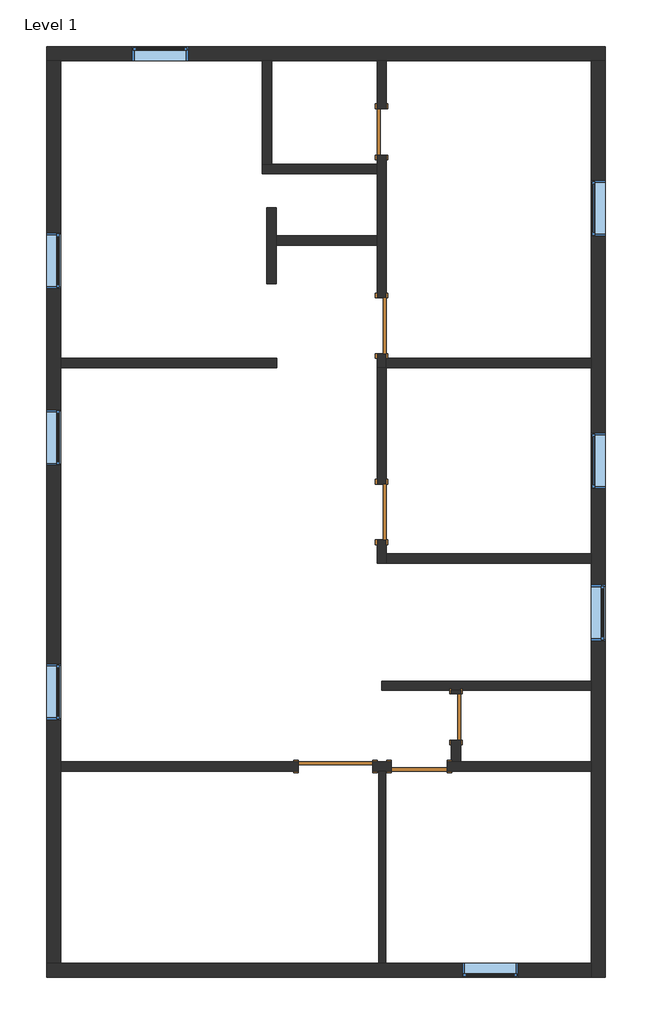
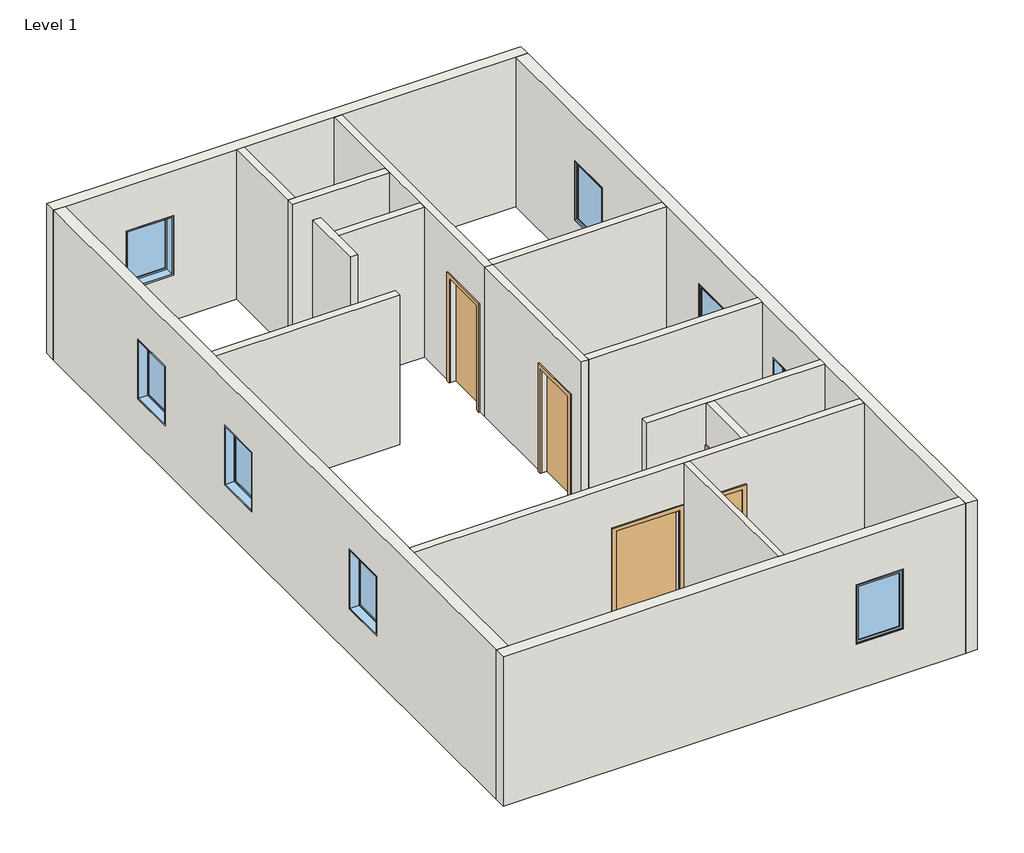
# One storey: 17 walls, 8 windows, 6 doors.
"""IFC4 building model written with IfcOpenShell, lengths in millimetres."""

from ifc_helpers import new_model, si_unit, frame, origin, origin_with_axes, place, context, project, spatial, polyline, outline, extrude, faceted_brep, transform, mapped, element, save
from components import door_e2b13fe9, door_16372e1c, door_3737b4f8, window_c1f32544

model = new_model("IFC4")

# Units and contexts
model_context = context("Model", 3, world=origin())
ifc_project = project(units=[si_unit("LENGTHUNIT", "METRE", prefix="MILLI")], contexts=[model_context])

# Site, building, storey
site = spatial("IfcSite", under=ifc_project)
building = spatial("IfcBuilding", under=site)
storey = spatial("IfcBuildingStorey", under=building, Name="Level 1", Elevation=0.0)

# Doors
placement = place(None, origin())
door_shape = door_e2b13fe9(model_context)
element("IfcDoor", 1, ObjectType="Single-Flush : 30\" x 84\"", at=placement, inside=storey, context=model_context, shape_type="MappedRepresentation", body=[
    mapped(door_shape, transform((-7001.2501883, 11107.9263771, 0.0), x_axis=(0.0, -1.0, 0.0), y_axis=(1.0, 0.0, 0.0), z_axis=(0.0, 0.0, 1.0))),
])
element("IfcDoor", 2, ObjectType="Single-Flush : 30\" x 84\"", at=placement, inside=storey, context=model_context, shape_type="MappedRepresentation", body=[
    mapped(door_shape, transform((-5782.0501883, 1532.1263771, 0.0), x_axis=(0.0, 1.0, 0.0), y_axis=(-1.0, 0.0, 0.0), z_axis=(0.0, 0.0, 1.0))),
])
door_2_shape = door_16372e1c(model_context)
element("IfcDoor", 3, ObjectType="Single-Flush : 36\" x 84\"", at=placement, inside=storey, context=model_context, shape_type="MappedRepresentation", body=[
    mapped(door_2_shape, transform((-7001.2501883, 7932.9263771, 0.0), x_axis=(0.0, -1.0, 0.0), y_axis=(1.0, 0.0, 0.0), z_axis=(0.0, 0.0, 1.0))),
])
element("IfcDoor", 4, ObjectType="Single-Flush : 36\" x 84\"", at=placement, inside=storey, context=model_context, shape_type="MappedRepresentation", body=[
    mapped(door_2_shape, transform((-7001.2501883, 4884.9263771, 0.0), x_axis=(0.0, -1.0, 0.0), y_axis=(1.0, 0.0, 0.0), z_axis=(0.0, 0.0, 1.0))),
])
element("IfcDoor", 5, ObjectType="Single-Flush : 36\" x 84\"", at=placement, inside=storey, context=model_context, shape_type="MappedRepresentation", body=[
    mapped(door_2_shape, transform((-6388.4751883, 719.3263771, 0.0), x_axis=(-1.0, 0.0, 0.0), y_axis=(0.0, -1.0, 0.0), z_axis=(0.0, 0.0, 1.0))),
])
door_3_shape = door_3737b4f8(model_context)
element("IfcDoor", 6, ObjectType="Single-Flush : 48\" x 84\"", at=placement, inside=storey, context=model_context, shape_type="MappedRepresentation", body=[
    mapped(door_3_shape, transform((-7756.9001883, 719.3263771, 0.0), x_axis=(-1.0, 0.0, 0.0), y_axis=(0.0, -1.0, 0.0), z_axis=(0.0, 0.0, 1.0))),
])

# Walls
element("IfcWall", 7, ObjectType="Generic - 4.5\"", at=placement, inside=storey, context=model_context, shape_type="SweptSolid", body=[
    extrude(outline(polyline([(-6937.7501883, 643.1263771), (-6937.7501883, -2506.4736229), (-7052.0501883, -2506.4736229), (-7052.0501883, 643.1263771), (-6937.7501883, 643.1263771)])), origin_with_axes(), (0.0, 0.0, 1.0), 3048.0),
])
element("IfcWall", 8, ObjectType="Generic - 6\"", at=placement, inside=storey, context=model_context, shape_type="Brep", body=[
    faceted_brep([(-7077.4501883, 7475.7263771, 2133.6), (-7077.4501883, 7475.7263771, 0.0), (-7077.4501883, 7247.1263771, 0.0), (-7077.4501883, 7247.1263771, 3048.0), (-7077.4501883, 9253.7263771, 3048.0), (-7077.4501883, 9406.1263771, 3048.0), (-7077.4501883, 10422.1263771, 3048.0), (-7077.4501883, 10574.5263771, 3048.0), (-7077.4501883, 12276.3263771, 3048.0), (-7077.4501883, 12276.3263771, 0.0), (-7077.4501883, 11488.9263771, 0.0), (-7077.4501883, 11488.9263771, 2133.6), (-7077.4501883, 10726.9263771, 2133.6), (-7077.4501883, 10726.9263771, 0.0), (-7077.4501883, 10574.5263771, 0.0), (-7077.4501883, 10422.1263771, 0.0), (-7077.4501883, 9406.1263771, 0.0), (-7077.4501883, 9253.7263771, 0.0), (-7077.4501883, 8390.1263771, 0.0), (-7077.4501883, 8390.1263771, 2133.6), (-6925.0501883, 7247.1263771, 0.0), (-6925.0501883, 7399.5263771, 0.0), (-6925.0501883, 7475.7263771, 0.0), (-6925.0501883, 7475.7263771, 2133.6), (-6925.0501883, 8390.1263771, 2133.6), (-6925.0501883, 8390.1263771, 0.0), (-6925.0501883, 10726.9263771, 0.0), (-6925.0501883, 10726.9263771, 2133.6), (-6925.0501883, 11488.9263771, 2133.6), (-6925.0501883, 11488.9263771, 0.0), (-6925.0501883, 12276.3263771, 0.0), (-6925.0501883, 12276.3263771, 3048.0), (-6925.0501883, 7399.5263771, 3048.0), (-6925.0501883, 7247.1263771, 3048.0)], [[[0, 1, 2, 3, 4, 5, 6, 7, 8, 9, 10, 11, 12, 13, 14, 15, 16, 17, 18, 19]], [[20, 21, 22, 23, 24, 25, 26, 27, 28, 29, 30, 31, 32, 33]], [[10, 9, 30, 29]], [[2, 1, 22, 21, 20]], [[18, 17, 16, 15, 14, 13, 26, 25]], [[8, 7, 6, 5, 4, 3, 33, 32, 31]], [[9, 8, 31, 30]], [[3, 2, 20, 33]], [[27, 26, 13, 12]], [[28, 27, 12, 11]], [[29, 28, 11, 10]], [[23, 22, 1, 0]], [[24, 23, 0, 19]], [[25, 24, 19, 18]]]),
])
element("IfcWall", 9, ObjectType="Generic - 6\"", at=placement, inside=storey, context=model_context, shape_type="SweptSolid", body=[
    extrude(outline(polyline([(-3572.2501883, 7247.1263771), (-6925.0501883, 7247.1263771), (-6925.0501883, 7399.5263771), (-3572.2501883, 7399.5263771), (-3572.2501883, 7247.1263771)])), origin_with_axes(), (0.0, 0.0, 1.0), 3048.0),
])
element("IfcWall", 10, ObjectType="Generic - 6\"", at=placement, inside=storey, context=model_context, shape_type="Brep", body=[
    faceted_brep([(-7077.4501883, 10574.5263771, 0.0), (-8804.6501883, 10574.5263771, 0.0), (-8957.0501883, 10574.5263771, 0.0), (-8957.0501883, 10574.5263771, 3048.0), (-8804.6501883, 10574.5263771, 3048.0), (-7077.4501883, 10574.5263771, 3048.0), (-7077.4501883, 10422.1263771, 0.0), (-7077.4501883, 10422.1263771, 3048.0), (-8957.0501883, 10422.1263771, 3048.0), (-8957.0501883, 10422.1263771, 0.0)], [[[0, 1, 2, 3, 4, 5]], [[6, 7, 8, 9]], [[2, 1, 0, 6, 9]], [[5, 4, 3, 8, 7]], [[0, 5, 7, 6]], [[3, 2, 9, 8]]]),
])
element("IfcWall", 11, ObjectType="Generic - 6\"", at=placement, inside=storey, context=model_context, shape_type="SweptSolid", body=[
    extrude(outline(polyline([(-8957.0501883, 10574.5263771), (-8957.0501883, 12276.3263771), (-8804.6501883, 12276.3263771), (-8804.6501883, 10574.5263771), (-8957.0501883, 10574.5263771)])), origin_with_axes(), (0.0, 0.0, 1.0), 3048.0),
])
element("IfcWall", 12, ObjectType="Generic - 6\"", at=placement, inside=storey, context=model_context, shape_type="SweptSolid", body=[
    extrude(outline(polyline([(-8728.4501883, 9406.1263771), (-7077.4501883, 9406.1263771), (-7077.4501883, 9253.7263771), (-8728.4501883, 9253.7263771), (-8728.4501883, 9406.1263771)])), origin_with_axes(), (0.0, 0.0, 1.0), 3048.0),
])
element("IfcWall", 13, ObjectType="Generic - 6\"", at=placement, inside=storey, context=model_context, shape_type="Brep", body=[
    faceted_brep([(-8728.4501883, 8618.7263771, 0.0), (-8728.4501883, 9253.7263771, 0.0), (-8728.4501883, 9406.1263771, 0.0), (-8728.4501883, 9863.3263771, 0.0), (-8728.4501883, 9863.3263771, 3048.0), (-8728.4501883, 9406.1263771, 3048.0), (-8728.4501883, 9253.7263771, 3048.0), (-8728.4501883, 8618.7263771, 3048.0), (-8880.8501883, 8618.7263771, 0.0), (-8880.8501883, 8618.7263771, 3048.0), (-8880.8501883, 9863.3263771, 3048.0), (-8880.8501883, 9863.3263771, 0.0)], [[[0, 1, 2, 3, 4, 5, 6, 7]], [[8, 9, 10, 11]], [[3, 2, 1, 0, 8, 11]], [[4, 3, 11, 10]], [[7, 6, 5, 4, 10, 9]], [[0, 7, 9, 8]]]),
])
element("IfcWall", 14, ObjectType="Generic - 6\"", at=placement, inside=storey, context=model_context, shape_type="SweptSolid", body=[
    extrude(outline(polyline([(-8715.7501883, 7247.1263771), (-12259.0501883, 7247.1263771), (-12259.0501883, 7399.5263771), (-8715.7501883, 7399.5263771), (-8715.7501883, 7247.1263771)])), origin_with_axes(), (0.0, 0.0, 1.0), 3048.0),
])
element("IfcWall", 15, ObjectType="Generic - 6\"", at=placement, inside=storey, context=model_context, shape_type="Brep", body=[
    faceted_brep([(-7077.4501883, 4427.7263771, 2133.6), (-7077.4501883, 4427.7263771, 0.0), (-7077.4501883, 4046.7263771, 0.0), (-7077.4501883, 4046.7263771, 3048.0), (-7077.4501883, 7247.1263771, 3048.0), (-7077.4501883, 7247.1263771, 0.0), (-7077.4501883, 5342.1263771, 0.0), (-7077.4501883, 5342.1263771, 2133.6), (-6925.0501883, 4046.7263771, 0.0), (-6925.0501883, 4199.1263771, 0.0), (-6925.0501883, 4427.7263771, 0.0), (-6925.0501883, 4427.7263771, 2133.6), (-6925.0501883, 5342.1263771, 2133.6), (-6925.0501883, 5342.1263771, 0.0), (-6925.0501883, 7247.1263771, 0.0), (-6925.0501883, 7247.1263771, 3048.0), (-6925.0501883, 4199.1263771, 3048.0), (-6925.0501883, 4046.7263771, 3048.0)], [[[0, 1, 2, 3, 4, 5, 6, 7]], [[8, 9, 10, 11, 12, 13, 14, 15, 16, 17]], [[6, 5, 14, 13]], [[2, 1, 10, 9, 8]], [[4, 3, 17, 16, 15]], [[5, 4, 15, 14]], [[3, 2, 8, 17]], [[11, 10, 1, 0]], [[12, 11, 0, 7]], [[13, 12, 7, 6]]]),
])
element("IfcWall", 16, ObjectType="Generic - 6\"", at=placement, inside=storey, context=model_context, shape_type="SweptSolid", body=[
    extrude(outline(polyline([(-3572.2501883, 4046.7263771), (-6925.0501883, 4046.7263771), (-6925.0501883, 4199.1263771), (-3572.2501883, 4199.1263771), (-3572.2501883, 4046.7263771)])), origin_with_axes(), (0.0, 0.0, 1.0), 3048.0),
])
element("IfcWall", 17, ObjectType="Generic - 6\"", at=placement, inside=storey, context=model_context, shape_type="Brep", body=[
    faceted_brep([(-7001.2501883, 1963.9263771, 0.0), (-5858.2501883, 1963.9263771, 0.0), (-5705.8501883, 1963.9263771, 0.0), (-3572.2501883, 1963.9263771, 0.0), (-3572.2501883, 1963.9263771, 3048.0), (-5705.8501883, 1963.9263771, 3048.0), (-5858.2501883, 1963.9263771, 3048.0), (-7001.2501883, 1963.9263771, 3048.0), (-7001.2501883, 2116.3263771, 0.0), (-7001.2501883, 2116.3263771, 3048.0), (-3572.2501883, 2116.3263771, 3048.0), (-3572.2501883, 2116.3263771, 0.0)], [[[0, 1, 2, 3, 4, 5, 6, 7]], [[8, 9, 10, 11]], [[3, 2, 1, 0, 8, 11]], [[7, 6, 5, 4, 10, 9]], [[0, 7, 9, 8]], [[4, 3, 11, 10]]]),
])
element("IfcWall", 18, ObjectType="Generic - 6\"", at=placement, inside=storey, context=model_context, shape_type="Brep", body=[
    faceted_brep([(-12259.0501883, 643.1263771, 0.0), (-8366.5001883, 643.1263771, 0.0), (-8366.5001883, 643.1263771, 2133.6), (-7147.3001883, 643.1263771, 2133.6), (-7147.3001883, 643.1263771, 0.0), (-7052.0501883, 643.1263771, 0.0), (-6937.7501883, 643.1263771, 0.0), (-6845.6751883, 643.1263771, 0.0), (-6845.6751883, 643.1263771, 2133.6), (-5931.2751883, 643.1263771, 2133.6), (-5931.2751883, 643.1263771, 0.0), (-3572.2501883, 643.1263771, 0.0), (-3572.2501883, 643.1263771, 3048.0), (-6937.7501883, 643.1263771, 3048.0), (-7052.0501883, 643.1263771, 3048.0), (-12259.0501883, 643.1263771, 3048.0), (-8366.5001883, 795.5263771, 2133.6), (-8366.5001883, 795.5263771, 0.0), (-12259.0501883, 795.5263771, 0.0), (-12259.0501883, 795.5263771, 3048.0), (-5858.2501883, 795.5263771, 3048.0), (-5705.8501883, 795.5263771, 3048.0), (-3572.2501883, 795.5263771, 3048.0), (-3572.2501883, 795.5263771, 0.0), (-5705.8501883, 795.5263771, 0.0), (-5858.2501883, 795.5263771, 0.0), (-5931.2751883, 795.5263771, 0.0), (-5931.2751883, 795.5263771, 2133.6), (-6845.6751883, 795.5263771, 2133.6), (-6845.6751883, 795.5263771, 0.0), (-7147.3001883, 795.5263771, 0.0), (-7147.3001883, 795.5263771, 2133.6)], [[[0, 1, 2, 3, 4, 5, 6, 7, 8, 9, 10, 11, 12, 13, 14, 15]], [[16, 17, 18, 19, 20, 21, 22, 23, 24, 25, 26, 27, 28, 29, 30, 31]], [[26, 25, 24, 23, 11, 10]], [[30, 29, 7, 6, 5, 4]], [[18, 17, 1, 0]], [[15, 14, 13, 12, 22, 21, 20, 19]], [[0, 15, 19, 18]], [[12, 11, 23, 22]], [[8, 7, 29, 28]], [[9, 8, 28, 27]], [[10, 9, 27, 26]], [[2, 1, 17, 16]], [[3, 2, 16, 31]], [[4, 3, 31, 30]]]),
])
element("IfcWall", 19, ObjectType="Generic - 6\"", at=placement, inside=storey, context=model_context, shape_type="SweptSolid", body=[
    extrude(outline(polyline([(1963.9263771, 0.0), (1913.1263771, 0.0), (1913.1263771, 2133.6), (1151.1263771, 2133.6), (1151.1263771, 0.0), (795.5263771, 0.0), (795.5263771, 3048.0), (1963.9263771, 3048.0), (1963.9263771, 0.0)])), frame((-5858.2501883, 0.0, 0.0), z_axis=(1.0, 0.0, 0.0), x_axis=(0.0, 1.0, 0.0)), (0.0, 0.0, 1.0), 152.4),
])
element("IfcWall", 20, ObjectType="Generic - 9\"", at=placement, inside=storey, context=model_context, shape_type="Brep", body=[
    faceted_brep([(-12487.6501883, 12276.3263771, 0.0), (-12259.0501883, 12276.3263771, 0.0), (-8957.0501883, 12276.3263771, 0.0), (-8804.6501883, 12276.3263771, 0.0), (-7077.4501883, 12276.3263771, 0.0), (-6925.0501883, 12276.3263771, 0.0), (-3572.2501883, 12276.3263771, 0.0), (-3343.6501883, 12276.3263771, 0.0), (-3343.6501883, 12276.3263771, 3048.0), (-3572.2501883, 12276.3263771, 3048.0), (-6925.0501883, 12276.3263771, 3048.0), (-7077.4501883, 12276.3263771, 3048.0), (-8804.6501883, 12276.3263771, 3048.0), (-8957.0501883, 12276.3263771, 3048.0), (-12259.0501883, 12276.3263771, 3048.0), (-12487.6501883, 12276.3263771, 3048.0), (-10169.9001883, 12276.3263771, 2133.6), (-10169.9001883, 12276.3263771, 914.4), (-11084.3001883, 12276.3263771, 914.4), (-11084.3001883, 12276.3263771, 2133.6), (-12487.6501883, 12504.9263771, 0.0), (-12487.6501883, 12504.9263771, 3048.0), (-3343.6501883, 12504.9263771, 3048.0), (-3343.6501883, 12504.9263771, 0.0), (-10169.9001883, 12504.9263771, 2133.6), (-11084.3001883, 12504.9263771, 2133.6), (-11084.3001883, 12504.9263771, 914.4), (-10169.9001883, 12504.9263771, 914.4)], [[[0, 1, 2, 3, 4, 5, 6, 7, 8, 9, 10, 11, 12, 13, 14, 15], [16, 17, 18, 19]], [[20, 21, 22, 23], [24, 25, 26, 27]], [[7, 6, 5, 4, 3, 2, 1, 0, 20, 23]], [[15, 14, 13, 12, 11, 10, 9, 8, 22, 21]], [[8, 7, 23, 22]], [[0, 15, 21, 20]], [[17, 16, 24, 27]], [[18, 17, 27, 26]], [[19, 18, 26, 25]], [[16, 19, 25, 24]]]),
])
element("IfcWall", 21, ObjectType="Generic - 9\"", at=placement, inside=storey, context=model_context, shape_type="Brep", body=[
    faceted_brep([(-3572.2501883, 12276.3263771, 0.0), (-3572.2501883, 7399.5263771, 0.0), (-3572.2501883, 7247.1263771, 0.0), (-3572.2501883, 4199.1263771, 0.0), (-3572.2501883, 4046.7263771, 0.0), (-3572.2501883, 2116.3263771, 0.0), (-3572.2501883, 1963.9263771, 0.0), (-3572.2501883, 795.5263771, 0.0), (-3572.2501883, 643.1263771, 0.0), (-3572.2501883, -2506.4736229, 0.0), (-3572.2501883, -2735.0736229, 0.0), (-3572.2501883, -2735.0736229, 3048.0), (-3572.2501883, -2506.4736229, 3048.0), (-3572.2501883, 643.1263771, 3048.0), (-3572.2501883, 795.5263771, 3048.0), (-3572.2501883, 1963.9263771, 3048.0), (-3572.2501883, 2116.3263771, 3048.0), (-3572.2501883, 4046.7263771, 3048.0), (-3572.2501883, 4199.1263771, 3048.0), (-3572.2501883, 7247.1263771, 3048.0), (-3572.2501883, 7399.5263771, 3048.0), (-3572.2501883, 12276.3263771, 3048.0), (-3572.2501883, 6180.3263771, 2133.6), (-3572.2501883, 5265.9263771, 2133.6), (-3572.2501883, 5265.9263771, 914.4), (-3572.2501883, 6180.3263771, 914.4), (-3572.2501883, 10314.1763771, 2133.6), (-3572.2501883, 9399.7763771, 2133.6), (-3572.2501883, 9399.7763771, 914.4), (-3572.2501883, 10314.1763771, 914.4), (-3572.2501883, 2776.7263771, 2133.6), (-3572.2501883, 2776.7263771, 914.4), (-3572.2501883, 3691.1263771, 914.4), (-3572.2501883, 3691.1263771, 2133.6), (-3343.6501883, 12276.3263771, 0.0), (-3343.6501883, 12276.3263771, 3048.0), (-3343.6501883, -2735.0736229, 3048.0), (-3343.6501883, -2735.0736229, 0.0), (-3343.6501883, 6180.3263771, 2133.6), (-3343.6501883, 6180.3263771, 914.4), (-3343.6501883, 5265.9263771, 914.4), (-3343.6501883, 5265.9263771, 2133.6), (-3343.6501883, 10314.1763771, 2133.6), (-3343.6501883, 10314.1763771, 914.4), (-3343.6501883, 9399.7763771, 914.4), (-3343.6501883, 9399.7763771, 2133.6), (-3343.6501883, 2776.7263771, 2133.6), (-3343.6501883, 3691.1263771, 2133.6), (-3343.6501883, 3691.1263771, 914.4), (-3343.6501883, 2776.7263771, 914.4)], [[[0, 1, 2, 3, 4, 5, 6, 7, 8, 9, 10, 11, 12, 13, 14, 15, 16, 17, 18, 19, 20, 21], [22, 23, 24, 25], [26, 27, 28, 29], [30, 31, 32, 33]], [[34, 35, 36, 37], [38, 39, 40, 41], [42, 43, 44, 45], [46, 47, 48, 49]], [[10, 9, 8, 7, 6, 5, 4, 3, 2, 1, 0, 34, 37]], [[21, 20, 19, 18, 17, 16, 15, 14, 13, 12, 11, 36, 35]], [[0, 21, 35, 34]], [[11, 10, 37, 36]], [[39, 38, 22, 25]], [[40, 39, 25, 24]], [[41, 40, 24, 23]], [[38, 41, 23, 22]], [[43, 42, 26, 29]], [[44, 43, 29, 28]], [[45, 44, 28, 27]], [[42, 45, 27, 26]], [[31, 30, 46, 49]], [[32, 31, 49, 48]], [[33, 32, 48, 47]], [[30, 33, 47, 46]]]),
])
element("IfcWall", 22, ObjectType="Generic - 9\"", at=placement, inside=storey, context=model_context, shape_type="Brep", body=[
    faceted_brep([(-3572.2501883, -2506.4736229, 0.0), (-6937.7501883, -2506.4736229, 0.0), (-7052.0501883, -2506.4736229, 0.0), (-12259.0501883, -2506.4736229, 0.0), (-12487.6501883, -2506.4736229, 0.0), (-12487.6501883, -2506.4736229, 3048.0), (-12259.0501883, -2506.4736229, 3048.0), (-7052.0501883, -2506.4736229, 3048.0), (-6937.7501883, -2506.4736229, 3048.0), (-3572.2501883, -2506.4736229, 3048.0), (-5683.6251883, -2506.4736229, 2133.6), (-5683.6251883, -2506.4736229, 914.4), (-4769.2251883, -2506.4736229, 914.4), (-4769.2251883, -2506.4736229, 2133.6), (-3572.2501883, -2735.0736229, 0.0), (-3572.2501883, -2735.0736229, 3048.0), (-12487.6501883, -2735.0736229, 3048.0), (-12487.6501883, -2735.0736229, 0.0), (-5683.6251883, -2735.0736229, 2133.6), (-4769.2251883, -2735.0736229, 2133.6), (-4769.2251883, -2735.0736229, 914.4), (-5683.6251883, -2735.0736229, 914.4)], [[[0, 1, 2, 3, 4, 5, 6, 7, 8, 9], [10, 11, 12, 13]], [[14, 15, 16, 17], [18, 19, 20, 21]], [[4, 3, 2, 1, 0, 14, 17]], [[9, 8, 7, 6, 5, 16, 15]], [[0, 9, 15, 14]], [[5, 4, 17, 16]], [[11, 10, 18, 21]], [[12, 11, 21, 20]], [[13, 12, 20, 19]], [[10, 13, 19, 18]]]),
])
element("IfcWall", 23, ObjectType="Generic - 9\"", at=placement, inside=storey, context=model_context, shape_type="Brep", body=[
    faceted_brep([(-12259.0501883, -2506.4736229, 0.0), (-12259.0501883, 643.1263771, 0.0), (-12259.0501883, 795.5263771, 0.0), (-12259.0501883, 7247.1263771, 0.0), (-12259.0501883, 7399.5263771, 0.0), (-12259.0501883, 12276.3263771, 0.0), (-12259.0501883, 12276.3263771, 3048.0), (-12259.0501883, 7399.5263771, 3048.0), (-12259.0501883, 7247.1263771, 3048.0), (-12259.0501883, 795.5263771, 3048.0), (-12259.0501883, 643.1263771, 3048.0), (-12259.0501883, -2506.4736229, 3048.0), (-12259.0501883, 8542.5263771, 2133.6), (-12259.0501883, 9456.9263771, 2133.6), (-12259.0501883, 9456.9263771, 914.4), (-12259.0501883, 8542.5263771, 914.4), (-12259.0501883, 5646.9263771, 2133.6), (-12259.0501883, 6561.3263771, 2133.6), (-12259.0501883, 6561.3263771, 914.4), (-12259.0501883, 5646.9263771, 914.4), (-12259.0501883, 1481.3263771, 2133.6), (-12259.0501883, 2395.7263771, 2133.6), (-12259.0501883, 2395.7263771, 914.4), (-12259.0501883, 1481.3263771, 914.4), (-12487.6501883, -2506.4736229, 0.0), (-12487.6501883, -2506.4736229, 3048.0), (-12487.6501883, 12276.3263771, 3048.0), (-12487.6501883, 12276.3263771, 0.0), (-12487.6501883, 8542.5263771, 2133.6), (-12487.6501883, 8542.5263771, 914.4), (-12487.6501883, 9456.9263771, 914.4), (-12487.6501883, 9456.9263771, 2133.6), (-12487.6501883, 5646.9263771, 2133.6), (-12487.6501883, 5646.9263771, 914.4), (-12487.6501883, 6561.3263771, 914.4), (-12487.6501883, 6561.3263771, 2133.6), (-12487.6501883, 1481.3263771, 2133.6), (-12487.6501883, 1481.3263771, 914.4), (-12487.6501883, 2395.7263771, 914.4), (-12487.6501883, 2395.7263771, 2133.6)], [[[0, 1, 2, 3, 4, 5, 6, 7, 8, 9, 10, 11], [12, 13, 14, 15], [16, 17, 18, 19], [20, 21, 22, 23]], [[24, 25, 26, 27], [28, 29, 30, 31], [32, 33, 34, 35], [36, 37, 38, 39]], [[5, 4, 3, 2, 1, 0, 24, 27]], [[11, 10, 9, 8, 7, 6, 26, 25]], [[0, 11, 25, 24]], [[6, 5, 27, 26]], [[29, 28, 12, 15]], [[30, 29, 15, 14]], [[31, 30, 14, 13]], [[28, 31, 13, 12]], [[33, 32, 16, 19]], [[34, 33, 19, 18]], [[35, 34, 18, 17]], [[32, 35, 17, 16]], [[37, 36, 20, 23]], [[38, 37, 23, 22]], [[39, 38, 22, 21]], [[36, 39, 21, 20]]]),
])

# Windows
window_shape = window_c1f32544(model_context)
element("IfcWindow", 24, ObjectType="Fixed : 36\" x 48\"", at=placement, inside=storey, context=model_context, shape_type="MappedRepresentation", body=[
    mapped(window_shape, transform((-10589.0001883, 12390.6263771, 0.0), x_axis=(1.0, 0.0, 0.0), y_axis=(0.0, 1.0, 0.0), z_axis=(0.0, 0.0, 1.0))),
])
element("IfcWindow", 25, ObjectType="Fixed : 36\" x 48\"", at=placement, inside=storey, context=model_context, shape_type="MappedRepresentation", body=[
    mapped(window_shape, transform((-12373.3501883, 8961.6263771, 0.0), x_axis=(0.0, -1.0, 0.0), y_axis=(1.0, 0.0, 0.0), z_axis=(0.0, 0.0, 1.0))),
])
element("IfcWindow", 26, ObjectType="Fixed : 36\" x 48\"", at=placement, inside=storey, context=model_context, shape_type="MappedRepresentation", body=[
    mapped(window_shape, transform((-12373.3501883, 6066.0263771, 0.0), x_axis=(0.0, -1.0, 0.0), y_axis=(1.0, 0.0, 0.0), z_axis=(0.0, 0.0, 1.0))),
])
element("IfcWindow", 27, ObjectType="Fixed : 36\" x 48\"", at=placement, inside=storey, context=model_context, shape_type="MappedRepresentation", body=[
    mapped(window_shape, transform((-12373.3501883, 1900.4263771, 0.0), x_axis=(0.0, -1.0, 0.0), y_axis=(1.0, 0.0, 0.0), z_axis=(0.0, 0.0, 1.0))),
])
element("IfcWindow", 28, ObjectType="Fixed : 36\" x 48\"", at=placement, inside=storey, context=model_context, shape_type="MappedRepresentation", body=[
    mapped(window_shape, transform((-3457.9501883, 5761.2263771, 0.0), x_axis=(0.0, 1.0, 0.0), y_axis=(-1.0, 0.0, 0.0), z_axis=(0.0, 0.0, 1.0))),
])
element("IfcWindow", 29, ObjectType="Fixed : 36\" x 48\"", at=placement, inside=storey, context=model_context, shape_type="MappedRepresentation", body=[
    mapped(window_shape, transform((-3457.9501883, 9895.0763771, 0.0), x_axis=(0.0, 1.0, 0.0), y_axis=(-1.0, 0.0, 0.0), z_axis=(0.0, 0.0, 1.0))),
])
element("IfcWindow", 30, ObjectType="Fixed : 36\" x 48\"", at=placement, inside=storey, context=model_context, shape_type="MappedRepresentation", body=[
    mapped(window_shape, transform((-3457.9501883, 3195.8263771, 0.0), x_axis=(0.0, -1.0, 0.0), y_axis=(1.0, 0.0, 0.0), z_axis=(0.0, 0.0, 1.0))),
])
element("IfcWindow", 31, ObjectType="Fixed : 36\" x 48\"", at=placement, inside=storey, context=model_context, shape_type="MappedRepresentation", body=[
    mapped(window_shape, transform((-5264.5251883, -2620.7736229, 0.0), x_axis=(-1.0, 0.0, 0.0), y_axis=(0.0, -1.0, 0.0), z_axis=(0.0, 0.0, 1.0))),
])

save(model, "model.ifc")

# Revit data of these elements
# Type "Single-Flush : 30\" x 84\""
#   Type Mark = "4"
#   Construction Type Id = "MDOOR"
#   Assembly Code = "C1020"
#   Analytic Construction = "Metal"
#   Thickness = 0' - 2"
#   Heat Transfer Coefficient (U) = 0.651978 BTU/(h·ft²·°F)
#   Height = 7' - 0"
#   Trim Projection Ext = 0' - 1"
#   Trim Projection Int = 0' - 1"
#   Trim Width = 0' - 3"
#   Width = 2' - 6"
#   Define Thermal Properties by = 1
#   Define Thermal Properties by = 1
#   Door Material = Door - Panel
#   Frame Material = Door - Frame
#   Visual Light Transmittance = 0
#   Solar Heat Gain Coefficient = 0
#   Function = (empty or 0)
#   Wall Closure = (empty or 0)
# Type "Single-Flush : 36\" x 84\""
#   Type Mark = "1"
#   Construction Type Id = "MDOOR"
#   Assembly Code = "C1020"
#   Analytic Construction = "Metal"
#   Thickness = 0' - 2"
#   Heat Transfer Coefficient (U) = 0.651978 BTU/(h·ft²·°F)
#   Height = 7' - 0"
#   Trim Projection Ext = 0' - 1"
#   Trim Projection Int = 0' - 1"
#   Trim Width = 0' - 3"
#   Width = 3' - 0"
#   Define Thermal Properties by = 1
#   Define Thermal Properties by = 1
#   Door Material = Door - Panel
#   Frame Material = Door - Frame
#   Visual Light Transmittance = 0
#   Solar Heat Gain Coefficient = 0
#   Function = (empty or 0)
#   Wall Closure = (empty or 0)
# Type "Single-Flush : 48\" x 84\""
#   Type Mark = "8"
#   Construction Type Id = "MDOOR"
#   Assembly Code = "C1020"
#   Analytic Construction = "Metal"
#   Thickness = 0' - 2"
#   Heat Transfer Coefficient (U) = 0.651978 BTU/(h·ft²·°F)
#   Height = 7' - 0"
#   Trim Projection Ext = 0' - 1"
#   Trim Projection Int = 0' - 1"
#   Trim Width = 0' - 3"
#   Width = 4' - 0"
#   Define Thermal Properties by = 1
#   Door Material = Door - Panel
#   Frame Material = Door - Frame
#   Visual Light Transmittance = 0
#   Solar Heat Gain Coefficient = 0
#   Function = (empty or 0)
#   Wall Closure = (empty or 0)
# Type "Generic - 4.5\""
#   Assembly Code = "B2010"
#   Layers, outside or top first: 0' - 4 1/2" no material (function 1)
# Type "Generic - 6\""
#   Assembly Code = "B2010"
#   Layers, outside or top first: 0' - 6" no material (function 1)
# Type "Generic - 9\""
#   Assembly Code = "B2010"
#   Layers, outside or top first: 0' - 9" "New Material" (function 1)
# Type "Fixed : 36\" x 48\""
#   Type Mark = "1"
#   Construction Type Id = "GSP4R"
#   Assembly Code = "B2020100"
#   Analytic Construction = "1/8 in Pilkington single glazing"
#   Visual Light Transmittance = 0.9
#   Solar Heat Gain Coefficient = 0.78
#   Heat Transfer Coefficient (U) = 0.6496 BTU/(h·ft²·°F)
#   Height = 4' - 0"
#   Default Sill Height = 3' - 0"
#   Width = 3' - 0"
#   Window Inset = 0' - 0 3/4"
#   Define Thermal Properties by = 1
#   Define Thermal Properties by = 1
#   Glass Pane Material = Glass
#   Sash Material = Sash
#   Wall Closure = (empty or 0)
# Elements 1, 2 (IfcDoor, "Single-Flush : 30\" x 84\"")
#   Phase Created = New Construction
#   Materials on its faces: "Door - Frame", "Door - Panel"
# Elements 3, 4, 5 (IfcDoor, "Single-Flush : 36\" x 84\"")
#   Phase Created = New Construction
#   Materials on its faces: "Door - Frame", "Door - Panel"
# Element 6 (IfcDoor, "Single-Flush : 48\" x 84\"")
#   Phase Created = New Construction
#   Materials on its faces: "Door - Frame", "Door - Panel"
# Element 7 (IfcWall, "Generic - 4.5\"")
#   Top Offset = 0' - 0"
#   Base Offset = 0' - 0"
#   wall height = 10' - 0"
#   Phase Created = New Construction
#   Base Constraint = Level 1
#   Top Constraint = Level 2
#   Materials on its faces: "Default Wall"
# Elements 8, 9, 10, 11, 12, 13, 14, 15, 16, 17, 18, 19 (IfcWall, "Generic - 6\"")
#   Top Offset = 0' - 0"
#   Base Offset = 0' - 0"
#   wall height = 10' - 0"
#   Phase Created = New Construction
#   Base Constraint = Level 1
#   Top Constraint = Level 2
#   Materials on its faces: "Default Wall"
# Elements 20, 21, 22, 23 (IfcWall, "Generic - 9\"")
#   Top Offset = 0' - 0"
#   Base Offset = 0' - 0"
#   wall height = 10' - 0"
#   Phase Created = New Construction
#   Base Constraint = Level 1
#   Top Constraint = Level 2
#   Materials on its faces: "New Material"
# Element 24 (IfcWindow, "Fixed : 36\" x 48\"")
#   Mark = "1"
#   Phase Created = New Construction
#   Materials on its faces: "Sash", "Glass"
# Element 25 (IfcWindow, "Fixed : 36\" x 48\"")
#   Mark = "2"
#   Phase Created = New Construction
#   Materials on its faces: "Sash", "Glass"
# Element 26 (IfcWindow, "Fixed : 36\" x 48\"")
#   Mark = "3"
#   Phase Created = New Construction
#   Materials on its faces: "Sash", "Glass"
# Element 27 (IfcWindow, "Fixed : 36\" x 48\"")
#   Mark = "4"
#   Phase Created = New Construction
#   Materials on its faces: "Sash", "Glass"
# Element 28 (IfcWindow, "Fixed : 36\" x 48\"")
#   Mark = "5"
#   Phase Created = New Construction
#   Materials on its faces: "Sash", "Glass"
# Element 29 (IfcWindow, "Fixed : 36\" x 48\"")
#   Mark = "6"
#   Phase Created = New Construction
#   Materials on its faces: "Sash", "Glass"
# Element 30 (IfcWindow, "Fixed : 36\" x 48\"")
#   Mark = "7"
#   Phase Created = New Construction
#   Materials on its faces: "Sash", "Glass"
# Element 31 (IfcWindow, "Fixed : 36\" x 48\"")
#   Mark = "8"
#   Phase Created = New Construction
#   Materials on its faces: "Sash", "Glass"
# Materials
#   "Door - Panel": class "Wood", colour RGB 210 159 95, transparency 0, Cost = 0
#   "Door - Frame": colour RGB 118 70 51, transparency 0, Cost = 0
#   "New Material": class "Generic", colour RGB 120 120 120, transparency 0, Cost = 0
#   "Glass": class "Glass", colour RGB 0 128 192, transparency 0.75, Description = "Soda Lime Glass", Cost = 0
#   "Sash": class "Wood", colour RGB 224 178 126, transparency 0, Cost = 0
#   "Default Wall": colour RGB 128 128 128, transparency 0, Cost = 0
